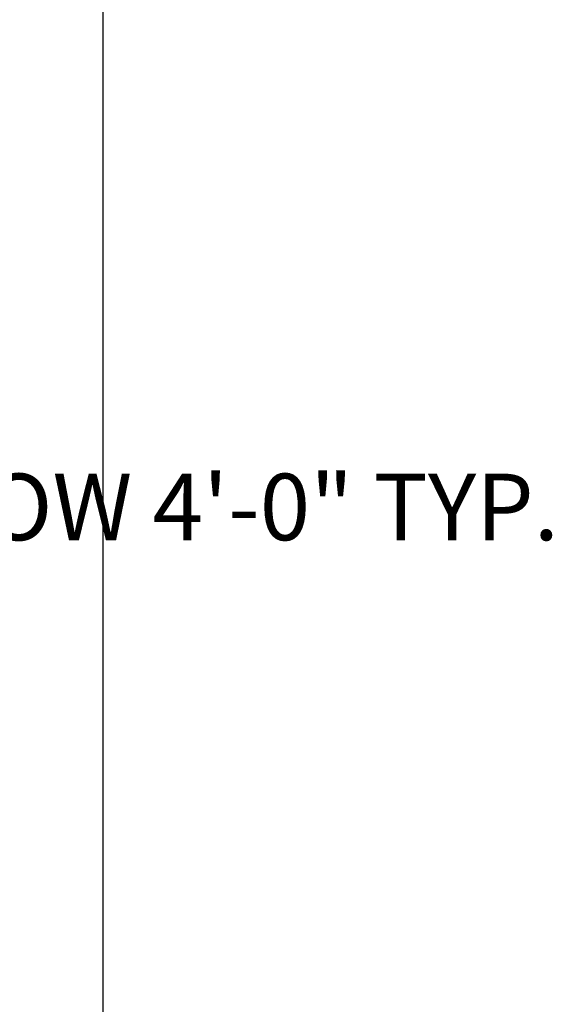
# Model space of a CAD drawing. Units: inches. Extents: x 528 to 2520, y -151 to 1354.
# Tile 26 of 41: x 1439 to 1487, y 1151 to 1239. Entities that reach past the tile are written whole.
import ezdxf

# ---------------------------------------------------------------- set-up
doc = ezdxf.new("R2010")
doc.units = ezdxf.units.IN
doc.header["$MEASUREMENT"] = 0
doc.layers.add('A-ANNO-DIMS', color=2, linetype='Continuous', lineweight=18)
doc.styles.get("Standard").update_dxf_attribs({"font": 'arial.ttf'})
doc.dimstyles.get("Standard").update_dxf_attribs({"dimtxt": 6, "dimasz": 2, "dimexe": 0.18, "dimexo": 0.0625, "dimgap": 0.09, "dimtad": 0, "dimtih": 1, "dimtoh": 1, "dimdec": 1, "dimzin": 0, "dimdsep": 46, "dimlunit": 3, "dimtxsty": 'Standard', "dimblk": 'ARCHTICK', "dimcen": 0.09, "dimadec": 0, "dimazin": 0, "dimtfac": 1, "dimtdec": 1, "dimtofl": 0, "dimtmove": 0, "dimatfit": 3, "dimfxl": 1, "dimtolj": 1, "dimtzin": 0, "dimarcsym": 0})

# ---------------------------------------------------------------- blocks, each defined once
blk = doc.blocks.new('_ArchTick')
at = {"color": 0, "linetype": 'ByBlock', "const_width": 0.15}
blk.add_lwpolyline([(-0.5, -0.5), (0.5, 0.5)], dxfattribs=at)
blk = doc.blocks.new('*D26')
at = {"layer": 'A-ANNO-DIMS', "color": 0, "lineweight": -2, "transparency": 16777216}
for p, q in [((1422.946, 1317.103), (1446.405, 1317.103)), ((1446.225, 1317.103), (1446.225, 1069.756)), ((1446.225, 816.103), (1446.225, 1063.449)), ((1422.946, 816.103), (1446.405, 816.103))]:
    blk.add_line(p, q, dxfattribs=at)
at = {"layer": 'Defpoints', "color": 0, "transparency": 16777216}
for p in [(1422.883, 1317.103), (1422.883, 816.103), (1446.225, 816.103)]:
    blk.add_point(p, dxfattribs=at)
at = {"layer": 'A-ANNO-DIMS', "color": 0, "lineweight": -2, "transparency": 16777216, "xscale": 2, "yscale": 2, "zscale": 2}
for p, rotation in [((1446.225, 1317.103), 90), ((1446.225, 816.103), 270)]:
    blk.add_blockref('_ArchTick', p, dxfattribs=dict(at, rotation=rotation))
at = {"layer": 'A-ANNO-DIMS', "color": 0, "transparency": 16777216, "insert": (1446.225, 1066.603), "char_height": 6, "attachment_point": 5}
blk.add_mtext('\\A1;41\'-9.0"', dxfattribs=at)
blk = doc.blocks.new('*D44')
at = {"layer": 'A-ANNO-DIMS', "color": 0, "lineweight": -2, "transparency": 16777216}
for p, q in [((1422.946, 1219.369), (1430.263, 1219.369)), ((1430.083, 1219.369), (1430.083, 1198.563)), ((1430.083, 1171.369), (1430.083, 1192.174)), ((1422.946, 1171.369), (1430.263, 1171.369))]:
    blk.add_line(p, q, dxfattribs=at)
at = {"layer": 'Defpoints', "color": 0, "transparency": 16777216}
for p in [(1422.883, 1219.369), (1430.083, 1219.369), (1422.883, 1171.369)]:
    blk.add_point(p, dxfattribs=at)
at = {"layer": 'A-ANNO-DIMS', "color": 0, "lineweight": -2, "transparency": 16777216, "xscale": 2, "yscale": 2, "zscale": 2}
for p, rotation in [((1430.083, 1219.369), 90), ((1430.083, 1171.369), 270)]:
    blk.add_blockref('_ArchTick', p, dxfattribs=dict(at, rotation=rotation))
at = {"layer": 'A-ANNO-DIMS', "color": 0, "transparency": 16777216, "insert": (1430.083, 1195.369), "char_height": 6, "attachment_point": 5}
blk.add_mtext('\\A1;BEDROOM WINDOW 4\'-0" TYP.', dxfattribs=at)

msp = doc.modelspace()

# ---------------------------------------------------------------- dimensions: what is measured, and where the dimension line sits
at = {"layer": 'A-ANNO-DIMS'}
dim = msp.add_linear_dim(base=(1446.225, 816.103), p1=(1422.883, 1317.103), p2=(1422.883, 816.103), angle=90, dimstyle='Standard', override={"dimclrd": 0, "dimclre": 0, "dimclrt": 0}, dxfattribs=at)
dim.commit()
dim.dimension.update_dxf_attribs({"geometry": '*D26', "text_midpoint": (1446.225, 1066.603)})
dim = msp.add_linear_dim(base=(1430.083, 1219.369), p1=(1422.883, 1171.369), p2=(1422.883, 1219.369), angle=90, text='BEDROOM WINDOW <> TYP.', dimstyle='Standard', override={"dimdec": 1, "dimlfac": 1, "dimrnd": 0, "dimzin": 1, "dimdsep": 46, "dimlunit": 4, "dimfrac": 2}, dxfattribs=at)
dim.commit()
dim.dimension.update_dxf_attribs({"geometry": '*D44', "text_midpoint": (1430.083, 1195.369)})

doc.saveas('drawing.dxf')
